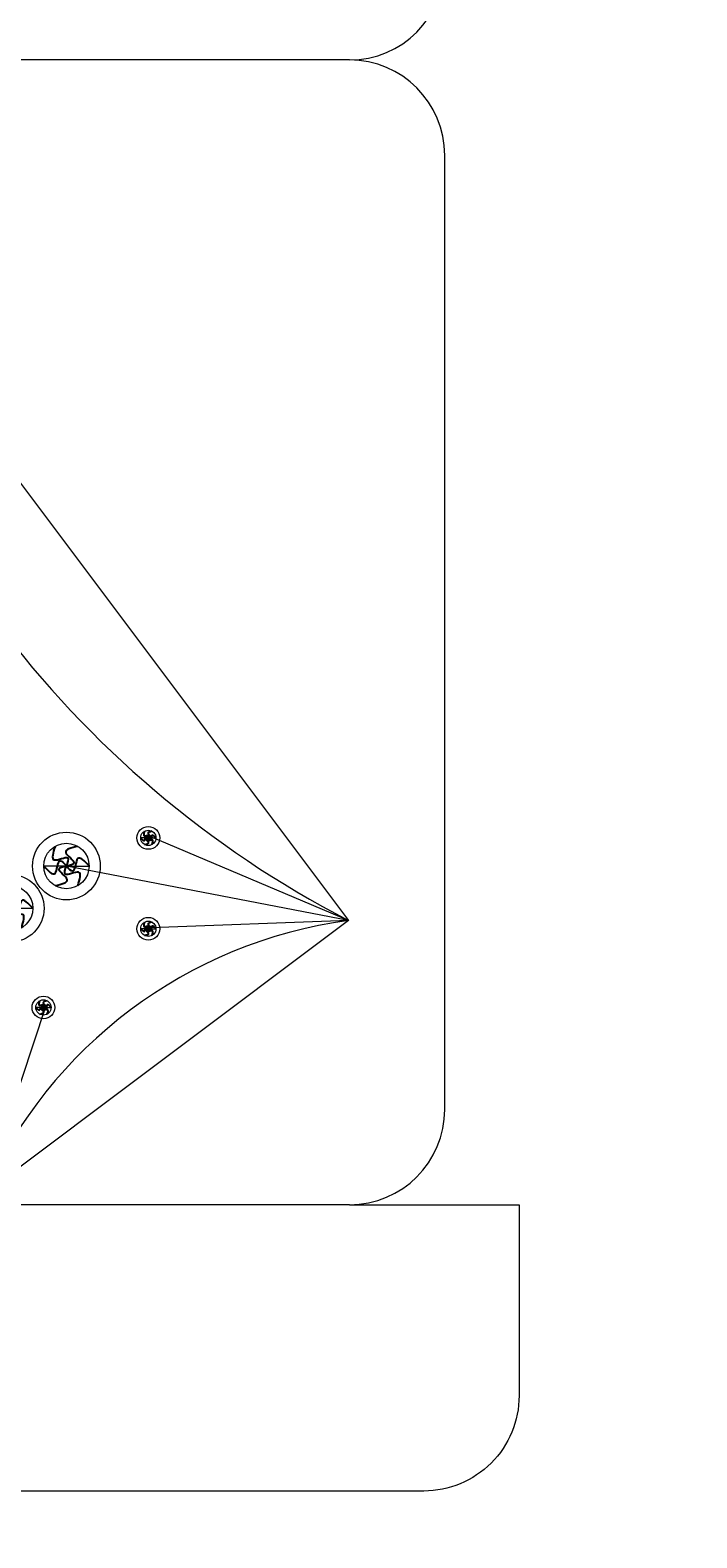
# Model space of a CAD drawing. Units: inches. Extents: x -61 to 1599, y -1316 to 257.
# Tile 104 of 204: x 142 to 156, y -131 to -99. Entities that reach past the tile are written whole.
import ezdxf

# ---------------------------------------------------------------- set-up
doc = ezdxf.new("R2010")
doc.units = ezdxf.units.IN
doc.header["$MEASUREMENT"] = 0
doc.layers.add('A-ANNO-DIMS', color=2, linetype='Continuous', lineweight=18)
doc.layers.add('FURNITURE', color=83, linetype='Continuous', lineweight=18)
doc.layers.add('FUR', color=83, linetype='Continuous')
doc.styles.get("Standard").update_dxf_attribs({"font": 'arial.ttf'})
doc.dimstyles.get("Standard").update_dxf_attribs({"dimtxt": 0.18, "dimasz": 0.18, "dimexe": 0.18, "dimexo": 0.0625, "dimgap": 0.09, "dimtad": 0, "dimtih": 1, "dimtoh": 1, "dimdec": 0, "dimzin": 0, "dimdsep": 46, "dimlunit": 3, "dimtxsty": 'Standard', "dimcen": 0.09, "dimadec": 0, "dimazin": 0, "dimtfac": 1, "dimtdec": 0, "dimtofl": 0, "dimtmove": 0, "dimatfit": 3, "dimfxl": 1, "dimtolj": 1, "dimtzin": 0, "dimarcsym": 0})

# ---------------------------------------------------------------- blocks, each defined once
blk = doc.blocks.new('*U183')
at = {"layer": 'FUR'}
blk.add_open_spline([(0.015, 0.238), (-0.088, 0.143), (-0.292, -0.045), (0.224, -0.053), (0.072, -0.187), (0.015, -0.238)], degree=3, knots=[0, 0, 0, 0, 0.2846533, 0.5662105, 0.736751, 0.736751, 0.736751, 0.736751], dxfattribs=at)
blk = doc.blocks.new('*U162')
at = {"layer": 'FUR', "transparency": 16777216}
for p, rotation in [((662.517, -238.489), 60), ((662.929, -238.463), 300), ((662.531, -238.727), 120), ((662.745, -238.833), 180), ((662.944, -238.702), 240)]:
    blk.add_blockref('*U183', p, dxfattribs=dict(at, rotation=rotation))
blk.add_blockref('*U183', (662.716, -238.357), dxfattribs=at)
blk = doc.blocks.new('*U182')
at = {"layer": 'FUR'}
blk.add_open_spline([(0.005, 0.08), (-0.03, 0.048), (-0.098, -0.015), (0.075, -0.018), (0.024, -0.063), (0.005, -0.08)], degree=3, knots=[0, 0, 0, 0, 0.0954578, 0.1898773, 0.2470677, 0.2470677, 0.2470677, 0.2470677], dxfattribs=at)
blk = doc.blocks.new('*U163')
at = {"layer": 'FUR', "transparency": 16777216}
for p, rotation in [((222.173, -79.977), 60), ((222.312, -79.968), 300), ((222.317, -80.048), 240), ((222.178, -80.056), 120), ((222.25, -80.092), 180)]:
    blk.add_blockref('*U182', p, dxfattribs=dict(at, rotation=rotation))
blk.add_blockref('*U182', (222.24, -79.932), dxfattribs=at)
blk = doc.blocks.new('*U166')
at = {"layer": 'FUR'}
blk.add_open_spline([(0.015, 0.238), (-0.088, 0.143), (-0.292, -0.045), (0.224, -0.053), (0.072, -0.187), (0.015, -0.238)], degree=3, knots=[0, 0, 0, 0, 0.2846533, 0.5662105, 0.736751, 0.736751, 0.736751, 0.736751], dxfattribs=at)
blk = doc.blocks.new('*U167')
at = {"layer": 'FUR', "transparency": 16777216}
for p, rotation in [((662.517, -238.489), 60), ((662.929, -238.463), 300), ((662.531, -238.727), 120), ((662.745, -238.833), 180), ((662.944, -238.702), 240)]:
    blk.add_blockref('*U166', p, dxfattribs=dict(at, rotation=rotation))
blk.add_blockref('*U166', (662.716, -238.357), dxfattribs=at)
blk = doc.blocks.new('*U178')
at = {"layer": 'FUR'}
blk.add_open_spline([(0.005, 0.08), (-0.03, 0.048), (-0.098, -0.015), (0.075, -0.018), (0.024, -0.063), (0.005, -0.08)], degree=3, knots=[0, 0, 0, 0, 0.0954578, 0.1898773, 0.2470677, 0.2470677, 0.2470677, 0.2470677], dxfattribs=at)
blk = doc.blocks.new('*U179')
at = {"layer": 'FUR', "transparency": 16777216}
for p, rotation in [((222.173, -79.977), 60), ((222.312, -79.968), 300), ((222.317, -80.048), 240), ((222.178, -80.056), 120), ((222.25, -80.092), 180)]:
    blk.add_blockref('*U178', p, dxfattribs=dict(at, rotation=rotation))
blk.add_blockref('*U178', (222.24, -79.932), dxfattribs=at)
blk = doc.blocks.new('*U180')
at = {"layer": 'FUR'}
blk.add_open_spline([(0.005, 0.08), (-0.03, 0.048), (-0.098, -0.015), (0.075, -0.018), (0.024, -0.063), (0.005, -0.08)], degree=3, knots=[0, 0, 0, 0, 0.0954578, 0.1898773, 0.2470677, 0.2470677, 0.2470677, 0.2470677], dxfattribs=at)
blk = doc.blocks.new('*U181')
at = {"layer": 'FUR', "transparency": 16777216}
for p, rotation in [((222.173, -79.977), 60), ((222.312, -79.968), 300), ((222.317, -80.048), 240), ((222.178, -80.056), 120), ((222.25, -80.092), 180)]:
    blk.add_blockref('*U180', p, dxfattribs=dict(at, rotation=rotation))
blk.add_blockref('*U180', (222.24, -79.932), dxfattribs=at)
blk = doc.blocks.new('SOFA-LOVESEAT')
for p, q in [((22.442, 30), (3.47, 30)), ((22.442, 30), (22.442, 30)), ((24.442, 8), (24.442, 28)), ((18.228, 13.691), (18.068, 13.691)), ((18.228, 13.691), (18.388, 13.691)), ((22.422, 11.961), (18.28, 13.711)), ((16.511, 13.102), (16.035, 13.102)), ((22.422, 11.961), (16.511, 13.102)), ((16.511, 13.102), (16.988, 13.102)), ((15.332, 12.217), (15.808, 12.217)), ((18.228, 11.787), (18.068, 11.787)), ((18.228, 11.787), (18.388, 11.787)), ((22.422, 11.961), (18.28, 11.807)), ((14.776, 6.223), (16.081, 10.156)), ((16.029, 10.137), (15.869, 10.137)), ((16.029, 10.137), (16.189, 10.137)), ((22.442, 6), (5.47, 6)), ((22.442, 6), (26, 6))]:
    blk.add_line(p, q)
blk.add_lwpolyline([(26, 6), (26, 2, -0.414214), (24, 0), (2, 0, -0.414214), (0, 2), (0, 58, -0.414213), (2, 60), (24, 60, -0.414214), (26, 58), (26, 54)], format="xyb")
blk.add_lwpolyline([(11.116, 27.026), (22.422, 11.961), (14.776, 6.223), (3.47, 21.288)], close=True)
for centre, radius in [((18.228, 13.691), 0.238), ((16.511, 13.102), 0.71), ((18.228, 13.691), 0.16), ((16.511, 13.102), 0.476), ((15.332, 12.217), 0.71), ((15.332, 12.217), 0.476), ((18.228, 11.787), 0.238), ((18.228, 11.787), 0.16), ((16.029, 10.137), 0.238), ((16.029, 10.137), 0.16)]:
    blk.add_circle(centre, radius)
for centre, radius, start, end in [((22.442, 32), 2, 270, 0), ((22.442, 28), 2, 0, 90), ((32.433, 31.248), 21.731, 191.2044, 242.5684), ((23.745, 2.234), 9.816, 97.747, 156.0258), ((22.442, 8), 2, 270, 0)]:
    blk.add_arc(centre, radius, start, end)
at = {"rotation": 90}
for name, p in [('*U167', (-222.084, -649.628)), ('*U181', (-61.785, -208.554)), ('*U162', (-223.264, -650.513)), ('*U179', (-61.785, -210.458)), ('*U163', (-63.983, -212.108))]:
    blk.add_blockref(name, p, dxfattribs=at)
blk = doc.blocks.new('*D687')
at = {"layer": 'A-ANNO-DIMS', "color": 0, "lineweight": -2, "transparency": 16777216}
for p, q in [((289.418, 181.677), (-61.077, 181.677)), ((-60.897, 181.497), (-60.897, -528.952)), ((-60.897, -1239.765), (-60.897, -529.316)), ((319.64, -1239.945), (-61.077, -1239.945))]:
    blk.add_line(p, q, dxfattribs=at)
at = {"layer": 'A-ANNO-DIMS', "color": 0, "transparency": 16777216}
for points in [[(-60.927, 181.497), (-60.867, 181.497), (-60.897, 181.677)], [(-60.927, -1239.765), (-60.867, -1239.765), (-60.897, -1239.945)]]:
    blk.add_solid(points, dxfattribs=at)
at = {"layer": 'DEFPOINTS', "color": 0, "transparency": 16777216}
for p in [(289.481, 181.677), (-60.897, -1239.945), (319.703, -1239.945)]:
    blk.add_point(p, dxfattribs=at)
at = {"layer": 'A-ANNO-DIMS', "color": 0, "transparency": 16777216, "insert": (-60.897, -529.134), "char_height": 0.18, "attachment_point": 5}
blk.add_mtext('\\A1;1421.6', dxfattribs=at)
blk = doc.blocks.new('*D700')
at = {"layer": 'A-ANNO-DIMS', "color": 0, "lineweight": -2, "transparency": 16777216}
for p, q in [((14.703, -616.882), (14.703, 257.457)), ((179.752, -616.882), (179.752, 257.457)), ((14.883, 257.277), (96.772, 257.277)), ((179.572, 257.277), (97.683, 257.277))]:
    blk.add_line(p, q, dxfattribs=at)
at = {"layer": 'A-ANNO-DIMS', "color": 0, "transparency": 16777216}
for points in [[(14.883, 257.307), (14.883, 257.247), (14.703, 257.277)], [(179.572, 257.307), (179.572, 257.247), (179.752, 257.277)]]:
    blk.add_solid(points, dxfattribs=at)
at = {"layer": 'DEFPOINTS', "color": 0, "transparency": 16777216}
for p in [(179.752, 257.277), (14.703, -616.945), (179.752, -616.945)]:
    blk.add_point(p, dxfattribs=at)
at = {"layer": 'A-ANNO-DIMS', "color": 0, "transparency": 16777216, "insert": (97.227, 257.277), "char_height": 0.18, "attachment_point": 5}
blk.add_mtext('\\A1;165.05', dxfattribs=at)

msp = doc.modelspace()

# ---------------------------------------------------------------- block references
at = {"layer": 'FURNITURE'}
msp.add_blockref('SOFA-LOVESEAT', (125.901, -129.695), dxfattribs=at)

# ---------------------------------------------------------------- dimensions: what is measured, and where the dimension line sits
at = {"layer": 'A-ANNO-DIMS'}
dim = msp.add_linear_dim(base=(179.7521, 257.2771), p1=(14.7028, -616.9446), p2=(179.7521, -616.9446), dimstyle='Standard', override={"dimdec": 2, "dimlfac": 1, "dimrnd": 0, "dimzin": 0, "dimdsep": 46, "dimlunit": 2}, dxfattribs=at)
dim.commit()
dim.dimension.update_dxf_attribs({"geometry": '*D700', "text_midpoint": (97.2274, 257.2771)})
dim = msp.add_linear_dim(base=(-60.8972, -1239.9446), p1=(289.4807, 181.6771), p2=(319.7028, -1239.9446), angle=90, dimstyle='Standard', override={"dimdec": 1, "dimlfac": 1, "dimrnd": 0, "dimzin": 0, "dimdsep": 46, "dimlunit": 2}, dxfattribs=at)
dim.commit()
dim.dimension.update_dxf_attribs({"geometry": '*D687', "text_midpoint": (-60.8972, -529.1337)})

doc.saveas('drawing.dxf')
